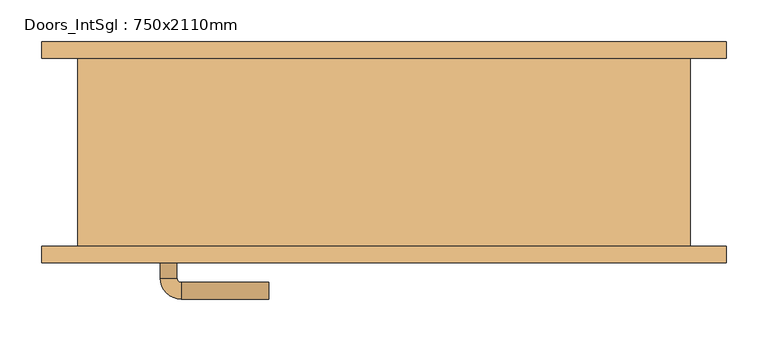
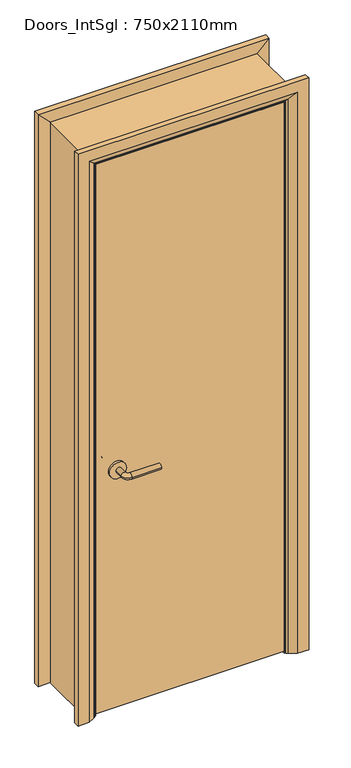
"""IFC4 building model written with IfcOpenShell, lengths in millimetres: door geometry, Doors_IntSgl : 750x2110mm."""

from ifc_helpers import new_model, si_unit, point, frame, frame_2d, origin, place, context, project, spatial, polyline, circle_curve, ellipse_curve, trimmed, segment, composite_curve, outline, extrude, faceted_brep, source, transform, mapped, element, save
from ifc_brep_helpers import plane_surface, cylinder_surface, revolved_surface, advanced_brep


def doors_intsgl_750x2110mm_8b4efb5c(model_context):
    return source(origin(), model_context, "Body", "SolidModel", [
        advanced_brep(
        [(-268.0, -66.5, 900.0), (-248.0, -66.5, 900.0), (-268.0, -36.5, 900.0), (-248.0, -36.5, 900.0), (-243.0, -31.5, 900.0), (-243.0, -11.5, 900.0), (-138.0, -11.5, 900.0), (-138.0, -31.5, 900.0)],
        [
            (0, 1, circle_curve(frame((-258.0, -66.5, 900.0), z_axis=(0.0, -1.0, 0.0), x_axis=(1.0, 0.0, 0.0)), 10.0)),
            (1, 0, circle_curve(frame((-258.0, -66.5, 900.0), z_axis=(0.0, -1.0, 0.0), x_axis=(1.0, 0.0, 0.0)), 10.0)),
            (0, 2),
            (2, 3, circle_curve(frame((-258.0, -36.5, 900.0), z_axis=(0.0, -1.0, 0.0), x_axis=(1.0, 0.0, 0.0)), 10.0)),
            (3, 1),
            (3, 2, circle_curve(frame((-258.0, -36.5, 900.0), z_axis=(0.0, -1.0, 0.0), x_axis=(1.0, 0.0, 0.0)), 10.0)),
            (4, 3, circle_curve(frame((-243.0, -36.5, 900.0), z_axis=(0.0, 0.0, 1.0), x_axis=(-1.0, 0.0, 0.0)), 5.0)),
            (2, 5, circle_curve(frame((-243.0, -36.5, 900.0), z_axis=(0.0, 0.0, -1.0), x_axis=(-1.0, 0.0, 0.0)), 25.0)),
            (5, 4, circle_curve(frame((-243.0, -21.5, 900.0), z_axis=(-1.0, 0.0, 0.0), x_axis=(0.0, -1.0, 0.0)), 10.0)),
            (4, 5, circle_curve(frame((-243.0, -21.5, 900.0), z_axis=(-1.0, 0.0, 0.0), x_axis=(0.0, -1.0, 0.0)), 10.0)),
            (6, 7, circle_curve(frame((-138.0, -21.5, 900.0), z_axis=(1.0, 0.0, 0.0), x_axis=(0.0, -1.0, 0.0)), 10.0)),
            (7, 6, circle_curve(frame((-138.0, -21.5, 900.0), z_axis=(1.0, 0.0, 0.0), x_axis=(0.0, -1.0, 0.0)), 10.0)),
            (5, 6),
            (7, 4),
        ],
        [
            plane_surface(frame((-258.0, -66.5, 900.0), z_axis=(0.0, -1.0, 0.0), x_axis=(0.0, 0.0, 1.0))),
            cylinder_surface(frame((-258.0, -66.5, 900.0), z_axis=(0.0, -1.0, 0.0), x_axis=(1.0, 0.0, 0.0)), 10.0),
            revolved_surface(trimmed(ellipse_curve(frame((-258.0, -36.5, 900.0), z_axis=(0.0, -1.0, 0.0), x_axis=(1.0, 0.0, 0.0)), 10.0, 10.0), [point((-268.0, -36.5, 900.0))], [point((-248.0, -36.5, 900.0))], True, "CARTESIAN"), (-243.0, -36.5, 900.0), (0.0, 0.0, -1.0)),
            revolved_surface(trimmed(ellipse_curve(frame((-258.0, -36.5, 900.0), z_axis=(0.0, -1.0, 0.0), x_axis=(1.0, 0.0, 0.0)), 10.0, 10.0), [point((-248.0, -36.5, 900.0))], [point((-268.0, -36.5, 900.0))], True, "CARTESIAN"), (-243.0, -36.5, 900.0), (0.0, 0.0, -1.0)),
            plane_surface(frame((-138.0, -21.5, 900.0), z_axis=(1.0, 0.0, 0.0), x_axis=(0.0, 0.0, 1.0))),
            cylinder_surface(frame((-243.0, -21.5, 900.0), z_axis=(-1.0, 0.0, 0.0), x_axis=(0.0, -1.0, 0.0)), 10.0),
        ],
        [
            (0, [[1, 2]]),
            (1, [[-1, 3, 4, 5]]),
            (1, [[-2, -5, 6, -3]]),
            (2, [[7, -4, 8, 9]]),
            (3, [[-8, -6, -7, 10]]),
            (4, [[11, 12]]),
            (5, [[-9, 13, -12, 14]]),
            (5, [[-10, -14, -11, -13]]),
        ],
    ),
        extrude(outline(composite_curve([segment(trimmed(circle_curve(frame_2d((900.0, -260.5)), 30.0), [point((900.0, -290.5))], [point((900.0, -230.5))], False, "CARTESIAN"), True, "CONTINUOUS"), segment(trimmed(circle_curve(frame_2d((900.0, -260.5)), 30.0), [point((900.0, -230.5))], [point((900.0, -290.5))], False, "CARTESIAN"), True, "CONTINUOUS")], self_intersect=False)), frame((0.0, -74.5, 0.0), z_axis=(0.0, 1.0, 0.0), x_axis=(0.0, 0.0, 1.0)), (0.0, 0.0, 1.0), 8.0),
        advanced_brep(
        [(-268.0, -120.5, 900.0), (-248.0, -120.5, 900.0), (-248.0, -150.5, 900.0), (-268.0, -150.5, 900.0), (-243.0, -155.5, 900.0), (-243.0, -175.5, 900.0), (-138.0, -175.5, 900.0), (-138.0, -155.5, 900.0)],
        [
            (0, 1, circle_curve(frame((-258.0, -120.5, 900.0), z_axis=(0.0, 1.0, 0.0), x_axis=(1.0, 0.0, 0.0)), 10.0)),
            (1, 0, circle_curve(frame((-258.0, -120.5, 900.0), z_axis=(0.0, 1.0, 0.0), x_axis=(1.0, 0.0, 0.0)), 10.0)),
            (1, 2),
            (2, 3, circle_curve(frame((-258.0, -150.5, 900.0), z_axis=(0.0, 1.0, 0.0), x_axis=(1.0, 0.0, 0.0)), 10.0)),
            (3, 0),
            (3, 2, circle_curve(frame((-258.0, -150.5, 900.0), z_axis=(0.0, 1.0, 0.0), x_axis=(1.0, 0.0, 0.0)), 10.0)),
            (4, 5, circle_curve(frame((-243.0, -165.5, 900.0), z_axis=(-1.0, 0.0, 0.0), x_axis=(0.0, 1.0, 0.0)), 10.0)),
            (5, 3, circle_curve(frame((-243.0, -150.5, 900.0), z_axis=(0.0, 0.0, -1.0), x_axis=(-1.0, 0.0, 0.0)), 25.0)),
            (2, 4, circle_curve(frame((-243.0, -150.5, 900.0), z_axis=(0.0, 0.0, 1.0), x_axis=(-1.0, 0.0, 0.0)), 5.0)),
            (5, 4, circle_curve(frame((-243.0, -165.5, 900.0), z_axis=(-1.0, 0.0, 0.0), x_axis=(0.0, 1.0, 0.0)), 10.0)),
            (6, 7, circle_curve(frame((-138.0, -165.5, 900.0), z_axis=(1.0, 0.0, 0.0), x_axis=(0.0, 1.0, 0.0)), 10.0)),
            (7, 6, circle_curve(frame((-138.0, -165.5, 900.0), z_axis=(1.0, 0.0, 0.0), x_axis=(0.0, 1.0, 0.0)), 10.0)),
            (4, 7),
            (6, 5),
        ],
        [
            plane_surface(frame((-258.0, -120.5, 900.0), z_axis=(0.0, 1.0, 0.0), x_axis=(0.0, 0.0, 1.0))),
            cylinder_surface(frame((-258.0, -120.5, 900.0), z_axis=(0.0, 1.0, 0.0), x_axis=(1.0, 0.0, 0.0)), 10.0),
            revolved_surface(trimmed(ellipse_curve(frame((-258.0, -150.5, 900.0), z_axis=(0.0, -1.0, 0.0), x_axis=(1.0, 0.0, 0.0)), 10.0, 10.0), [point((-268.0, -150.5, 900.0))], [point((-248.0, -150.5, 900.0))], True, "CARTESIAN"), (-243.0, -150.5, 900.0), (0.0, 0.0, -1.0)),
            revolved_surface(trimmed(ellipse_curve(frame((-258.0, -150.5, 900.0), z_axis=(0.0, -1.0, 0.0), x_axis=(1.0, 0.0, 0.0)), 10.0, 10.0), [point((-248.0, -150.5, 900.0))], [point((-268.0, -150.5, 900.0))], True, "CARTESIAN"), (-243.0, -150.5, 900.0), (0.0, 0.0, -1.0)),
            plane_surface(frame((-138.0, -165.5, 900.0), z_axis=(1.0, 0.0, 0.0), x_axis=(0.0, 0.0, 1.0))),
            cylinder_surface(frame((-243.0, -165.5, 900.0), z_axis=(-1.0, 0.0, 0.0), x_axis=(0.0, 1.0, 0.0)), 10.0),
        ],
        [
            (0, [[1, 2]]),
            (1, [[3, 4, 5, -2]]),
            (1, [[-5, 6, -3, -1]]),
            (2, [[7, 8, -4, 9]]),
            (3, [[10, -9, -6, -8]]),
            (4, [[11, 12]]),
            (5, [[13, -11, 14, -7]]),
            (5, [[-14, -12, -13, -10]]),
        ],
    ),
        extrude(outline(composite_curve([segment(trimmed(circle_curve(frame_2d((900.0, -260.5)), 30.0), [point((900.0, -290.5))], [point((900.0, -230.5))], False, "CARTESIAN"), True, "CONTINUOUS"), segment(trimmed(circle_curve(frame_2d((900.0, -260.5)), 30.0), [point((900.0, -230.5))], [point((900.0, -290.5))], False, "CARTESIAN"), True, "CONTINUOUS")], self_intersect=False)), frame((0.0, -120.5, 0.0), z_axis=(0.0, 1.0, 0.0), x_axis=(0.0, 0.0, 1.0)), (0.0, 0.0, 1.0), 8.0),
        extrude(outline(polyline([(333.0, -74.5), (333.0, -112.5), (-333.0, -112.5), (-333.0, -74.5), (333.0, -74.5)])), frame((0.0, 0.0, 8.0), z_axis=(0.0, 0.0, 1.0), x_axis=(1.0, 0.0, 0.0)), (0.0, 0.0, 1.0), 2060.0),
        advanced_brep(
        [(410.0, -132.5, 0.0), (370.0, -132.5, 0.0), (344.0, -118.5, 0.0), (340.0, -112.5, 0.0), (410.0, -112.5, 0.0), (410.0, -112.5, 2145.0), (410.0, -132.5, 2145.0), (340.0, -112.5, 2075.0), (-340.0, -112.5, 2075.0), (-340.0, -112.5, 0.0), (-410.0, -112.5, 0.0), (-410.0, -112.5, 2145.0), (344.0, -118.5, 2079.0), (370.0, -132.5, 2105.0), (-410.0, -132.5, 2145.0), (-410.0, -132.5, 0.0), (-370.0, -132.5, 0.0), (-370.0, -132.5, 2105.0), (-344.0, -118.5, 2079.0), (-344.0, -118.5, 0.0)],
        [
            (0, 1),
            (1, 2),
            (2, 3, circle_curve(frame((348.0, -111.5, 0.0), z_axis=(0.0, 0.0, -1.0), x_axis=(1.0, 0.0, 0.0)), 8.0622577)),
            (3, 4),
            (4, 0),
            (4, 5),
            (5, 6),
            (6, 0),
            (3, 7),
            (7, 8),
            (8, 9),
            (9, 10),
            (10, 11),
            (11, 5),
            (2, 12),
            (12, 7, ellipse_curve(frame((348.0, -111.5, 2083.0), z_axis=(0.7071067811865475, 0.0, -0.7071067811865475), x_axis=(-0.7071067811865474, 0.0, -0.7071067811865476)), 11.4017543, 8.0622577)),
            (1, 13),
            (13, 12),
            (6, 14),
            (14, 15),
            (15, 16),
            (16, 17),
            (17, 13),
            (11, 14),
            (12, 18),
            (18, 8, ellipse_curve(frame((-348.0, -111.5, 2083.0), z_axis=(0.7071067811865475, 0.0, 0.7071067811865475), x_axis=(0.7071067811865476, 0.0, -0.7071067811865474)), 11.4017543, 8.0622577)),
            (17, 18),
            (15, 10),
            (9, 19, circle_curve(frame((-348.0, -111.5, 0.0), z_axis=(0.0, 0.0, -1.0), x_axis=(-1.0, 0.0, 0.0)), 8.0622577)),
            (19, 16),
            (18, 19),
        ],
        [
            plane_surface(frame((340.0, -112.5, 0.0), z_axis=(0.0, 0.0, -1.0), x_axis=(0.0, 1.0, 0.0))),
            plane_surface(frame((410.0, -132.5, 0.0), z_axis=(1.0, 0.0, 0.0), x_axis=(0.0, 0.0, 1.0))),
            plane_surface(frame((410.0, -112.5, 0.0), z_axis=(0.0, 1.0, 0.0), x_axis=(0.0, 0.0, 1.0))),
            cylinder_surface(frame((348.0, -111.5, 0.0), z_axis=(0.0, 0.0, -1.0), x_axis=(1.0, 0.0, 0.0)), 8.0622577),
            plane_surface(frame((344.0, -118.5, 0.0), z_axis=(-0.4740998230350126, -0.880471099922178, 0.0), x_axis=(0.0, 0.0, 1.0))),
            plane_surface(frame((370.0, -132.5, 0.0), z_axis=(0.0, -1.0, 0.0), x_axis=(0.0, 0.0, 1.0))),
            plane_surface(frame((410.0, -132.5, 2145.0), z_axis=(0.0, 0.0, 1.0), x_axis=(-1.0, 0.0, 0.0))),
            cylinder_surface(frame((340.0, -111.5, 2083.0), z_axis=(1.0, 0.0, 0.0), x_axis=(0.0, 0.0, 1.0)), 8.0622577),
            plane_surface(frame((344.0, -118.5, 2079.0), z_axis=(0.0, -0.8804710999221764, -0.4740998230350154), x_axis=(-1.0, 0.0, 0.0))),
            plane_surface(frame((-340.0, -112.5, 0.0), z_axis=(0.0, 0.0, -1.0), x_axis=(0.0, 1.0, 0.0))),
            plane_surface(frame((-410.0, -132.5, 2145.0), z_axis=(-1.0, 0.0, 0.0), x_axis=(0.0, 0.0, -1.0))),
            cylinder_surface(frame((-348.0, -111.5, 2075.0), z_axis=(0.0, 0.0, 1.0), x_axis=(-1.0, 0.0, 0.0)), 8.0622577),
            plane_surface(frame((-344.0, -118.5, 2079.0), z_axis=(0.47409982303501824, -0.8804710999221749, 0.0), x_axis=(0.0, 0.0, -1.0))),
        ],
        [
            (0, [[1, 2, 3, 4, 5]]),
            (1, [[6, 7, 8, -5]]),
            (2, [[9, 10, 11, 12, 13, 14, -6, -4]]),
            (3, [[15, 16, -9, -3]]),
            (4, [[17, 18, -15, -2]]),
            (5, [[-8, 19, 20, 21, 22, 23, -17, -1]]),
            (6, [[-14, 24, -19, -7]]),
            (7, [[25, 26, -10, -16]]),
            (8, [[-23, 27, -25, -18]]),
            (9, [[28, -12, 29, 30, -21]]),
            (10, [[-13, -28, -20, -24]]),
            (11, [[31, -29, -11, -26]]),
            (12, [[-22, -30, -31, -27]]),
        ],
    ),
        extrude(outline(polyline([(0.0, -316.0), (2051.0, -316.0), (2051.0, 316.0), (0.0, 316.0), (0.0, 335.0), (2070.0, 335.0), (2070.0, -335.0), (0.0, -335.0), (0.0, -316.0)])), frame((0.0, -72.5, 0.0), z_axis=(0.0, 1.0, 0.0), x_axis=(0.0, 0.0, 1.0)), (0.0, 0.0, 1.0), 32.0),
        advanced_brep(
        [(-410.0, 132.5, 0.0), (-370.0, 132.5, 0.0), (-344.0, 118.5, 0.0), (-340.0, 112.5, 0.0), (-410.0, 112.5, 0.0), (-410.0, 112.5, 2145.0), (-410.0, 132.5, 2145.0), (-340.0, 112.5, 2075.0), (-344.0, 118.5, 2079.0), (-370.0, 132.5, 2105.0), (410.0, 112.5, 2145.0), (410.0, 132.5, 2145.0), (340.0, 112.5, 2075.0), (344.0, 118.5, 2079.0), (370.0, 132.5, 2105.0), (410.0, 132.5, 0.0), (410.0, 112.5, 0.0), (340.0, 112.5, 0.0), (344.0, 118.5, 0.0), (370.0, 132.5, 0.0)],
        [
            (0, 1),
            (1, 2),
            (2, 3, circle_curve(frame((-348.0, 111.5, 0.0), z_axis=(0.0, 0.0, -1.0), x_axis=(-1.0, 0.0, 0.0)), 8.0622577)),
            (3, 4),
            (4, 0),
            (4, 5),
            (5, 6),
            (6, 0),
            (3, 7),
            (7, 5),
            (2, 8),
            (8, 7, ellipse_curve(frame((-348.0, 111.5, 2083.0), z_axis=(-0.7071067811865475, 0.0, -0.7071067811865475), x_axis=(0.7071067811865474, 0.0, -0.7071067811865476)), 11.4017543, 8.0622577)),
            (1, 9),
            (9, 8),
            (6, 9),
            (5, 10),
            (10, 11),
            (11, 6),
            (7, 12),
            (12, 10),
            (8, 13),
            (13, 12, ellipse_curve(frame((348.0, 111.5, 2083.0), z_axis=(-0.7071067811865475, 0.0, 0.7071067811865475), x_axis=(-0.7071067811865476, 0.0, -0.7071067811865474)), 11.4017543, 8.0622577)),
            (9, 14),
            (14, 13),
            (11, 14),
            (15, 16),
            (16, 17),
            (17, 18, circle_curve(frame((348.0, 111.5, 0.0), z_axis=(0.0, 0.0, -1.0), x_axis=(1.0, 0.0, 0.0)), 8.0622577)),
            (18, 19),
            (19, 15),
            (10, 16),
            (15, 11),
            (12, 17),
            (13, 18),
            (14, 19),
        ],
        [
            plane_surface(frame((-340.0, 185.3010989, 0.0), z_axis=(0.0, 0.0, -1.0), x_axis=(1.0, 0.0, 0.0))),
            plane_surface(frame((-410.0, 132.5, 0.0), z_axis=(-1.0, 0.0, 0.0), x_axis=(0.0, 0.0, 1.0))),
            plane_surface(frame((-410.0, 112.5, 0.0), z_axis=(0.0, -1.0, 0.0), x_axis=(0.0, 0.0, 1.0))),
            cylinder_surface(frame((-348.0, 111.5, 0.0), z_axis=(0.0, 0.0, -1.0), x_axis=(-1.0, 0.0, 0.0)), 8.0622577),
            plane_surface(frame((-344.0, 118.5, 0.0), z_axis=(0.4740998230350183, 0.8804710999221749, 0.0), x_axis=(0.0, 0.0, 1.0))),
            plane_surface(frame((-370.0, 132.5, 0.0), z_axis=(0.0, 1.0, 0.0), x_axis=(0.0, 0.0, 1.0))),
            plane_surface(frame((-410.0, 132.5, 2145.0), z_axis=(0.0, 0.0, 1.0), x_axis=(1.0, 0.0, 0.0))),
            plane_surface(frame((-410.0, 112.5, 2145.0), z_axis=(0.0, -1.0, 0.0), x_axis=(1.0, 0.0, 0.0))),
            cylinder_surface(frame((-340.0, 111.5, 2083.0), z_axis=(-1.0, 0.0, 0.0), x_axis=(0.0, 0.0, 1.0)), 8.0622577),
            plane_surface(frame((-344.0, 118.5, 2079.0), z_axis=(0.0, 0.8804710999221749, -0.4740998230350183), x_axis=(1.0, 0.0, 0.0))),
            plane_surface(frame((-370.0, 132.5, 2105.0), z_axis=(0.0, 1.0, 0.0), x_axis=(1.0, 0.0, 0.0))),
            plane_surface(frame((340.0, 185.3010989, 0.0), z_axis=(0.0, 0.0, -1.0), x_axis=(-1.0, 0.0, 0.0))),
            plane_surface(frame((410.0, 132.5, 2145.0), z_axis=(1.0, 0.0, 0.0), x_axis=(0.0, 0.0, -1.0))),
            plane_surface(frame((410.0, 112.5, 2145.0), z_axis=(0.0, -1.0, 0.0), x_axis=(0.0, 0.0, -1.0))),
            cylinder_surface(frame((348.0, 111.5, 2075.0), z_axis=(0.0, 0.0, 1.0), x_axis=(1.0, 0.0, 0.0)), 8.0622577),
            plane_surface(frame((344.0, 118.5, 2079.0), z_axis=(-0.4740998230350183, 0.8804710999221749, 0.0), x_axis=(0.0, 0.0, -1.0))),
            plane_surface(frame((370.0, 132.5, 2105.0), z_axis=(0.0, 1.0, 0.0), x_axis=(0.0, 0.0, -1.0))),
        ],
        [
            (0, [[1, 2, 3, 4, 5]]),
            (1, [[6, 7, 8, -5]]),
            (2, [[9, 10, -6, -4]]),
            (3, [[11, 12, -9, -3]]),
            (4, [[13, 14, -11, -2]]),
            (5, [[-8, 15, -13, -1]]),
            (6, [[16, 17, 18, -7]]),
            (7, [[19, 20, -16, -10]]),
            (8, [[21, 22, -19, -12]]),
            (9, [[23, 24, -21, -14]]),
            (10, [[-18, 25, -23, -15]]),
            (11, [[26, 27, 28, 29, 30]]),
            (12, [[31, -26, 32, -17]]),
            (13, [[33, -27, -31, -20]]),
            (14, [[34, -28, -33, -22]]),
            (15, [[35, -29, -34, -24]]),
            (16, [[-32, -30, -35, -25]]),
        ],
    ),
        faceted_brep([(-335.0, -112.5, 0.0), (-367.0, -112.5, 0.0), (-367.0, 112.5, 0.0), (-335.0, 112.5, 0.0), (-335.0, 112.5, 2070.0), (-335.0, -112.5, 2070.0), (-367.0, 112.5, 2102.0), (-367.0, -112.5, 2102.0), (335.0, 112.5, 2070.0), (335.0, -112.5, 2070.0), (367.0, 112.5, 2102.0), (367.0, -112.5, 2102.0), (335.0, -112.5, 0.0), (335.0, 112.5, 0.0), (367.0, 112.5, 0.0), (367.0, -112.5, 0.0)], [[[0, 1, 2, 3]], [[3, 4, 5, 0]], [[2, 6, 4, 3]], [[1, 7, 6, 2]], [[0, 5, 7, 1]], [[4, 8, 9, 5]], [[6, 10, 8, 4]], [[7, 11, 10, 6]], [[5, 9, 11, 7]], [[12, 13, 14, 15]], [[8, 13, 12, 9]], [[10, 14, 13, 8]], [[11, 15, 14, 10]], [[9, 12, 15, 11]]]),
    ])


if __name__ == "__main__":
    model = new_model("IFC4")
    model_context = context("Model", 3, world=origin())
    ifc_project = project(units=[si_unit("LENGTHUNIT", "METRE", prefix="MILLI")], contexts=[model_context])
    site = spatial("IfcSite", under=ifc_project)
    building = spatial("IfcBuilding", under=site)
    placement = place(None, origin())
    doors_intsgl_750x2110mm_shape = doors_intsgl_750x2110mm_8b4efb5c(model_context)
    element("IfcDoor", 1, ObjectType="Doors_IntSgl : 750x2110mm", at=placement, inside=building, context=model_context, shape_type="MappedRepresentation", body=[
        mapped(doors_intsgl_750x2110mm_shape, transform((0.0, 0.0, 0.0), x_axis=(1.0, 0.0, 0.0), y_axis=(0.0, 1.0, 0.0), z_axis=(0.0, 0.0, 1.0))),
    ])
    save(model, "model.ifc")

# Revit data of these elements
# Type "Doors_IntSgl : 750x2110mm"
#   Construction Type Id = "MDOOR"
#   Type Mark = "42"
#   Type Comments = "Internal Single"
#   Operation = "SingleSwingRight"
#   Manufacturer = "Revit"
#   Keynote = "L20"
#   Description = "Internal Single Door"
#   Analytic Construction = "Metal"
#   UnderCut = 8 mm
#   Tolerance = 2 mm
#   Thickness = 38 mm
#   Thermal Resistance (R) = 0.270117 (m²·K)/W
#   Structural Tolerance = 8 mm
#   StopDepth = 32 mm
#   Stop Thickness = 19 mm
#   Rough Width = 750 mm
#   Rough Height = 2110 mm
#   Height to Top Lock Rail = 1000 mm
#   Heat Transfer Coefficient (U) = 3.7021 W/(m²·K)
#   Handle Z Distance = 900 mm
#   Handle X Distance = 75 mm
#   Frame Thickness = 32 mm
#   Door Panel Width = 666 mm
#   Door Panel Thickness = 38 mm
#   Door Panel Offset = 0 mm
#   Height = 2110 mm
#   Width = 750 mm
#   Door Panel Height = 2060 mm
#   Architrave Setback = 5 mm
#   Define Thermal Properties by = 1
#   Vis - Ironmongery = yes
#   Material Ironmongery = Door - Handle
#   Material Frame = Door - Frame/Mullion (1)
#   Material Door = Door - Panel
#   Material Architrave = Door - Architrave
#   Visual Light Transmittance = 0
#   Solar Heat Gain Coefficient = 0
#   Function = (empty or 0)
#   Wall Closure = (empty or 0)
# Element 1 (IfcDoor, "Doors_IntSgl : 750x2110mm")
#   Materials on its faces: "Door - Architrave", "Door - Handle", "Door - Frame/Mullion (1)", "Door - Panel"
# Materials
#   "Door - Handle": colour RGB 0 0 0, transparency 0, Keynote = "P21", Cost = 0
#   "Door - Frame/Mullion (1)": class "Wood", colour RGB 212 179 113, transparency 0, Keynote = "L20", Cost = 0
#   "Door - Panel": class "Wood", colour RGB 210 159 95, transparency 0, Keynote = "L20", Cost = 0
#   "Door - Architrave": class "Wood", colour RGB 154 90 5, transparency 0, Keynote = "P20", Cost = 0
